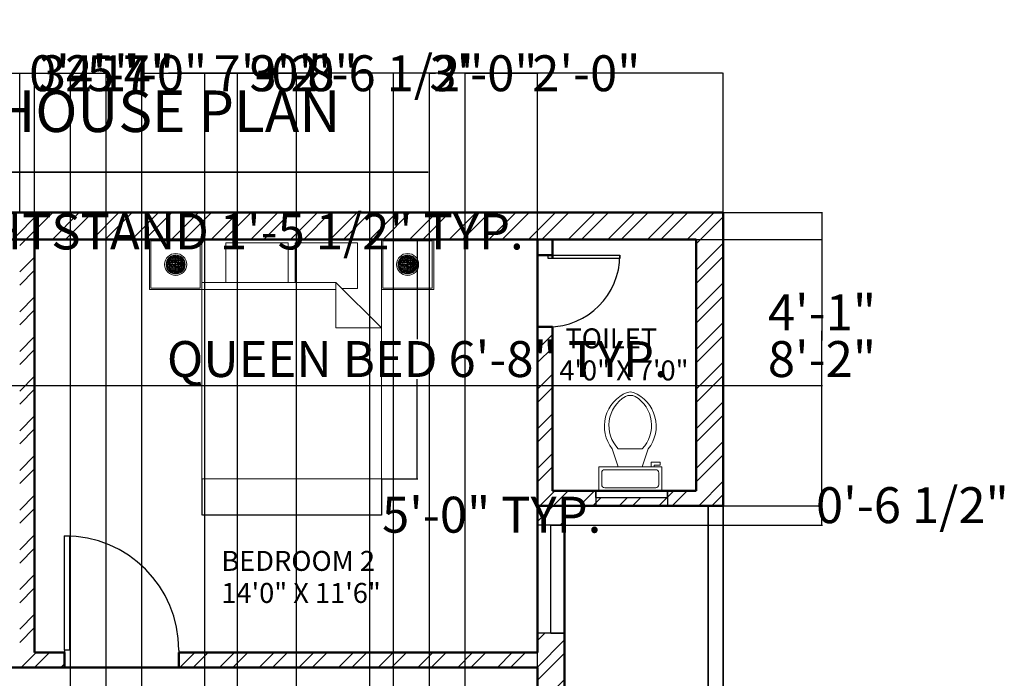
# Model space of a CAD drawing. Units: inches. Extents: x -40 to 578, y -482 to 237.
# Tile 7 of 7: x 249 to 578, y 17 to 237. Entities that reach past the tile are written whole.
import ezdxf

# ---------------------------------------------------------------- set-up
doc = ezdxf.new("R2010")
doc.units = ezdxf.units.IN
doc.header["$MEASUREMENT"] = 0
for name, color, linetype, lineweight in [('A-ANNO-DIMS', 2, 'Continuous', 18), ('A-ANNO-TEXT', 7, 'Continuous', 35), ('A-AREA-IDEN', 240, 'Continuous', 25), ('A-FLOR-FIXT', 4, 'Continuous', 18), ('A-FURN', 4, 'Continuous', 18), ('A-WALL-PATT', 252, 'Continuous', 13), ('C-PROP', 3, 'Continuous', 35), ('DOORS', 2, 'Continuous', 25), ('WALLS', 3, 'Continuous', 50), ('WINDOWS', 241, 'Continuous', 25)]:
    doc.layers.add(name, color=color, linetype=linetype, lineweight=lineweight)
doc.styles.get("Standard").update_dxf_attribs({"font": 'arial.ttf'})
doc.dimstyles.get("Standard").update_dxf_attribs({"dimtxt": 12, "dimasz": 0.18, "dimexe": 0.18, "dimexo": 0.0625, "dimgap": 0.09, "dimtad": 0, "dimtih": 1, "dimtoh": 1, "dimdec": 0, "dimzin": 0, "dimdsep": 46, "dimlunit": 3, "dimtxsty": 'Standard', "dimcen": 0.09, "dimadec": 0, "dimazin": 0, "dimtfac": 1, "dimtdec": 0, "dimtofl": 0, "dimtmove": 0, "dimatfit": 3, "dimfxl": 1, "dimtolj": 1, "dimtzin": 0, "dimarcsym": 0})

# ---------------------------------------------------------------- blocks, each defined once
blk = doc.blocks.new('Bed - Queen')
for p, q in [((0, -80.00003), (0, 0)), ((0, 0), (59.99999, 0)), ((59.99999, 0), (59.99999, -80.00003)), ((7.99999, -1.2), (28.79998, -1.2)), ((7.99999, -14.4), (7.99999, -1.2)), ((28.79998, -1.2), (28.79998, -14.4)), ((31.19999, -1.2), (51.99999, -1.2)), ((31.19999, -14.4), (31.19999, -1.2)), ((51.99999, -1.2), (51.99999, -16.4)), ((0, -14.4), (44.8, -14.4)), ((59.99999, -29.6), (44.8, -14.4)), ((44.8, -14.4), (44.8, -29.6)), ((51.99999, -16.4), (46.79936, -16.4)), ((44.8, -16.8), (0, -16.8)), ((44.8, -29.6), (59.99999, -29.6)), ((59.99999, -80.00003), (0, -80.00003))]:
    blk.add_line(p, q)
blk = doc.blocks.new('Toilet - top')
for p, q in [((9.5, -6), (9.5, -2)), ((-10, -8.5), (-8, -8.5)), ((-10, -9.5), (-10, -8.5)), ((-7, -9.5), (-10, -9.5)), ((-8, -8.5), (-8, -8)), ((-7, -8), (-7, -9.5)), ((-4, -8), (-6, -14)), ((4, -8), (6, -14)), ((4, -14), (-4, -14))]:
    blk.add_line(p, q)
blk.add_lwpolyline([(10.5, -8), (10.5, 0), (-10.5, 0), (-10.5, -8)], close=True)
for points in [[(-9.5, -2), (-9.5, -6)], [(8.5, -1), (-8.5, -1)], [(-8.5, -7), (8.5, -7)]]:
    blk.add_lwpolyline(points)
for centre, radius, start, end in [((-8.62, -1.88), 0.884, 81.8699, 188.1301), ((8.62, -1.88), 0.884, 351.8699, 98.1301), ((-8.62, -6.12), 0.884, 171.8699, 278.1301), ((8.62, -6.12), 0.884, 261.8699, 8.1301), ((3.52, -21.58), 12.17, 141.4691, 247.9714), ((4.2, -21.82), 11.33, 136.3677, 238.9468), ((-3.52, -21.58), 12.17, 292.0284, 38.5307), ((-4.2, -21.82), 11.33, 301.053, 43.6321), ((0, -27.88), 4, 245.7318, 294.2682), ((0, -29), 4, 254.8605, 285.1395)]:
    blk.add_arc(centre, radius, start, end)
blk = doc.blocks.new('*U10')
for p, q in [((0, 0), (0, -6)), ((40, 0), (40, -6))]:
    blk.add_line(p, q)
blk.add_lwpolyline([(0, 0), (0, 40), (1.75, 40), (1.75, 0)], close=True)
blk.add_arc((0, 0), 40, 0, 90)
blk = doc.blocks.new('NIGHTSTAND-LAMP')
for p, q in [((6.65, 10.79), (5.56, 8.46)), ((7.17, 11.17), (5.64, 7.78)), ((6.14, 10.22), (5.64, 9.09)), ((7.58, 11.36), (5.82, 7.16)), ((8.24, 11.54), (6.14, 6.59)), ((6.14, 10.22), (11.36, 10.22)), ((6.14, 10.22), (6.14, 6.58)), ((6.5, 10.65), (10.99, 10.65)), ((8.75, 11.58), (6.65, 6.01)), ((6.65, 10.79), (6.65, 6.01)), ((9.21, 11.55), (7.17, 5.63)), ((7.17, 11.17), (10.32, 11.17)), ((7.17, 11.17), (7.17, 5.63)), ((9.71, 11.43), (7.58, 5.44)), ((7.58, 11.36), (7.58, 5.44)), ((8.24, 11.54), (8.24, 5.18)), ((10.22, 11.22), (8.24, 5.26)), ((8.75, 11.58), (8.75, 5.22)), ((10.75, 10.87), (8.75, 5.22)), ((9.21, 11.55), (9.21, 5.18)), ((10.99, 10.65), (9.21, 5.18)), ((9.71, 11.43), (9.71, 5.37)), ((11.15, 10.48), (9.71, 5.37)), ((10.22, 11.22), (10.22, 5.58)), ((11.36, 10.22), (10.22, 5.58)), ((10.75, 10.87), (10.75, 5.93)), ((11.15, 10.48), (11.15, 6.31)), ((5.56, 8.4), (11.93, 8.4)), ((5.63, 7.78), (11.87, 7.78)), ((5.64, 9.09), (11.85, 9.09)), ((5.64, 9.09), (5.64, 7.71)), ((5.82, 7.16), (11.68, 7.16)), ((5.83, 9.68), (11.66, 9.68)), ((6.13, 6.59), (11.37, 6.59)), ((11.66, 9.68), (10.75, 5.93)), ((11.85, 9.09), (11.15, 6.31)), ((11.81, 9.26), (11.81, 7.54)), ((6.6, 6.05), (10.9, 6.05)), ((7.18, 5.63), (10.31, 5.63))]:
    blk.add_line(p, q)
for points in [[(17.49, 16.8), (0, 16.8), (0, 0), (17.49, 0)], [(16.99, 16.3), (0.5, 16.3), (0.5, 0.5), (16.99, 0.5)]]:
    blk.add_lwpolyline(points, close=True)
for radius in [3.68, 3.18]:
    blk.add_circle((8.75, 8.4), radius)
blk = doc.blocks.new('WIN-36IN')
for p, q in [((9, 36), (0, 36)), ((4.5, 0), (4.5, 36)), ((4.5, 36), (9, 36)), ((9, 0), (0, 0)), ((4.5, 0), (9, 0))]:
    blk.add_line(p, q)
blk = doc.blocks.new('*D28')
at = {"layer": 'A-ANNO-DIMS', "color": 0, "lineweight": -2, "transparency": 16777216}
for p, q in [((188.56, 163.51), (188.56, 166.25)), ((188.74, 166.07), (205.87, 166.07)), ((206.05, 163.51), (206.05, 166.25)), ((206.05, 166.07), (206.23, 166.07))]:
    blk.add_line(p, q, dxfattribs=at)
at = {"layer": 'A-ANNO-DIMS', "color": 0, "transparency": 16777216}
for points in [[(188.74, 166.1), (188.74, 166.04), (188.56, 166.07)], [(205.87, 166.1), (205.87, 166.04), (206.05, 166.07)]]:
    blk.add_solid(points, dxfattribs=at)
at = {"layer": 'Defpoints', "color": 0, "transparency": 16777216}
for p in [(206.05, 166.07), (188.56, 163.45), (206.05, 163.45)]:
    blk.add_point(p, dxfattribs=at)
at = {"layer": 'A-ANNO-DIMS', "color": 0, "transparency": 16777216, "insert": (313.4, 166.07), "char_height": 12, "attachment_point": 5}
blk.add_mtext('\\A1;NIGHTSTAND 1\'-5 1/2" TYP.', dxfattribs=at)
blk = doc.blocks.new('*D32')
at = {"layer": 'A-ANNO-DIMS', "color": 0, "lineweight": -2, "transparency": 16777216}
for p, q in [((369.65, 163.45), (381.77, 163.45)), ((381.59, 163.27), (381.59, 130.11)), ((381.59, 83.63), (381.59, 116.78)), ((369.65, 83.45), (381.77, 83.45))]:
    blk.add_line(p, q, dxfattribs=at)
at = {"layer": 'A-ANNO-DIMS', "color": 0, "transparency": 16777216}
for points in [[(381.56, 163.27), (381.62, 163.27), (381.59, 163.45)], [(381.56, 83.63), (381.62, 83.63), (381.59, 83.45)]]:
    blk.add_solid(points, dxfattribs=at)
at = {"layer": 'Defpoints', "color": 0, "transparency": 16777216}
for p in [(369.59, 163.45), (381.59, 163.45), (369.59, 83.45)]:
    blk.add_point(p, dxfattribs=at)
at = {"layer": 'A-ANNO-DIMS', "color": 0, "transparency": 16777216, "insert": (381.59, 123.45), "char_height": 12, "attachment_point": 5}
blk.add_mtext('\\A1;QUEEN BED 6\'-8" TYP.', dxfattribs=at)
blk = doc.blocks.new('*D33')
at = {"layer": 'A-ANNO-DIMS', "color": 0, "lineweight": -2, "transparency": 16777216}
for p, q in [((309.59, 83.38), (309.59, 71.27)), ((369.59, 83.38), (369.59, 71.27)), ((309.77, 71.45), (369.41, 71.45)), ((369.59, 71.45), (369.77, 71.45))]:
    blk.add_line(p, q, dxfattribs=at)
at = {"layer": 'A-ANNO-DIMS', "color": 0, "transparency": 16777216}
for points in [[(309.77, 71.48), (309.77, 71.42), (309.59, 71.45)], [(369.41, 71.48), (369.41, 71.42), (369.59, 71.45)]]:
    blk.add_solid(points, dxfattribs=at)
at = {"layer": 'Defpoints', "color": 0, "transparency": 16777216}
for p in [(309.59, 83.45), (369.59, 83.45), (369.59, 71.45)]:
    blk.add_point(p, dxfattribs=at)
at = {"layer": 'A-ANNO-DIMS', "color": 0, "transparency": 16777216, "insert": (406.43, 71.45), "char_height": 12, "attachment_point": 5}
blk.add_mtext('\\A1;5\'-0" TYP.', dxfattribs=at)
blk = doc.blocks.new('*D45')
at = {"layer": 'A-ANNO-DIMS', "color": 0, "lineweight": -2, "transparency": 16777216}
for p, q in [((71.74, 172.51), (71.74, 219.12)), ((71.92, 218.94), (257.04, 218.94)), ((483.56, 218.94), (298.43, 218.94)), ((483.74, 172.51), (483.74, 219.12))]:
    blk.add_line(p, q, dxfattribs=at)
at = {"layer": 'A-ANNO-DIMS', "color": 0, "transparency": 16777216}
for points in [[(71.92, 218.97), (71.92, 218.91), (71.74, 218.94)], [(483.56, 218.97), (483.56, 218.91), (483.74, 218.94)]]:
    blk.add_solid(points, dxfattribs=at)
at = {"layer": 'Defpoints', "color": 0, "transparency": 16777216}
for p in [(483.74, 218.94), (71.74, 172.45), (483.74, 172.45)]:
    blk.add_point(p, dxfattribs=at)
at = {"layer": 'A-ANNO-DIMS', "color": 0, "transparency": 16777216, "insert": (277.74, 218.94), "char_height": 12, "attachment_point": 5}
blk.add_mtext('\\A1;34\'-4"', dxfattribs=at)
blk = doc.blocks.new('*D46')
at = {"layer": 'A-ANNO-DIMS', "color": 0, "lineweight": -2, "transparency": 16777216}
for p, q in [((483.8, 172.45), (516.97, 172.45)), ((516.79, 172.27), (516.79, 129.66)), ((516.79, 74.63), (516.79, 117.23)), ((483.8, 74.45), (516.97, 74.45))]:
    blk.add_line(p, q, dxfattribs=at)
at = {"layer": 'A-ANNO-DIMS', "color": 0, "transparency": 16777216}
for points in [[(516.76, 172.27), (516.82, 172.27), (516.79, 172.45)], [(516.76, 74.63), (516.82, 74.63), (516.79, 74.45)]]:
    blk.add_solid(points, dxfattribs=at)
at = {"layer": 'Defpoints', "color": 0, "transparency": 16777216}
for p in [(483.74, 172.45), (516.79, 172.45), (483.74, 74.45)]:
    blk.add_point(p, dxfattribs=at)
at = {"layer": 'A-ANNO-DIMS', "color": 0, "transparency": 16777216, "insert": (516.79, 123.45), "char_height": 12, "attachment_point": 5}
blk.add_mtext('\\A1;8\'-2"', dxfattribs=at)
blk = doc.blocks.new('*D49')
at = {"layer": 'A-ANNO-DIMS', "color": 0, "lineweight": -2, "transparency": 16777216}
for p, q in [((385.66, -377.49), (385.66, 219.12)), ((385.84, 218.94), (387.66, 218.94)), ((421.56, 218.94), (419.73, 218.94)), ((421.74, -377.49), (421.74, 219.12))]:
    blk.add_line(p, q, dxfattribs=at)
at = {"layer": 'A-ANNO-DIMS', "color": 0, "transparency": 16777216}
for points in [[(385.84, 218.97), (385.84, 218.91), (385.66, 218.94)], [(421.56, 218.97), (421.56, 218.91), (421.74, 218.94)]]:
    blk.add_solid(points, dxfattribs=at)
at = {"layer": 'Defpoints', "color": 0, "transparency": 16777216}
for p in [(421.74, 218.94), (385.66, -377.55), (421.74, -377.55)]:
    blk.add_point(p, dxfattribs=at)
at = {"layer": 'A-ANNO-DIMS', "color": 0, "transparency": 16777216, "insert": (403.7, 218.94), "char_height": 12, "attachment_point": 5}
blk.add_mtext('\\A1;3\'-0"', dxfattribs=at)
blk = doc.blocks.new('*D50')
at = {"layer": 'A-ANNO-DIMS', "color": 0, "lineweight": -2, "transparency": 16777216}
for p, q in [((265.66, -330.99), (265.66, 219.12)), ((265.84, 218.94), (277.48, 218.94)), ((277.66, -330.99), (277.66, 219.12)), ((277.66, 218.94), (277.84, 218.94))]:
    blk.add_line(p, q, dxfattribs=at)
at = {"layer": 'A-ANNO-DIMS', "color": 0, "transparency": 16777216}
for points in [[(265.84, 218.97), (265.84, 218.91), (265.66, 218.94)], [(277.48, 218.97), (277.48, 218.91), (277.66, 218.94)]]:
    blk.add_solid(points, dxfattribs=at)
at = {"layer": 'Defpoints', "color": 0, "transparency": 16777216}
for p in [(277.66, 218.94), (265.66, -331.05), (277.66, -331.05)]:
    blk.add_point(p, dxfattribs=at)
at = {"layer": 'A-ANNO-DIMS', "color": 0, "transparency": 16777216, "insert": (293.31, 218.94), "char_height": 12, "attachment_point": 5}
blk.add_mtext('\\A1;1\'-0"', dxfattribs=at)
blk = doc.blocks.new('*D52')
at = {"layer": 'A-ANNO-DIMS', "color": 0, "lineweight": -2, "transparency": 16777216}
for p, q in [((234.57, -377.49), (234.57, 219.12)), ((234.75, 218.94), (265.48, 218.94)), ((265.66, -377.49), (265.66, 219.12)), ((265.66, 218.94), (265.84, 218.94))]:
    blk.add_line(p, q, dxfattribs=at)
at = {"layer": 'A-ANNO-DIMS', "color": 0, "transparency": 16777216}
for points in [[(234.75, 218.97), (234.75, 218.91), (234.57, 218.94)], [(265.48, 218.97), (265.48, 218.91), (265.66, 218.94)]]:
    blk.add_solid(points, dxfattribs=at)
at = {"layer": 'Defpoints', "color": 0, "transparency": 16777216}
for p in [(265.66, 218.94), (234.57, -377.55), (265.66, -377.55)]:
    blk.add_point(p, dxfattribs=at)
at = {"layer": 'A-ANNO-DIMS', "color": 0, "transparency": 16777216, "insert": (281.98, 218.94), "char_height": 12, "attachment_point": 5}
blk.add_mtext('\\A1;2\'-7"', dxfattribs=at)
blk = doc.blocks.new('*D61')
at = {"layer": 'A-ANNO-DIMS', "color": 0, "lineweight": -2, "transparency": 16777216}
for p, q in [((248.74, 172.51), (248.74, 219.12)), ((248.92, 218.94), (253.56, 218.94)), ((253.74, 172.51), (253.74, 219.12)), ((253.74, 218.94), (253.92, 218.94))]:
    blk.add_line(p, q, dxfattribs=at)
at = {"layer": 'A-ANNO-DIMS', "color": 0, "transparency": 16777216}
for points in [[(248.92, 218.97), (248.92, 218.91), (248.74, 218.94)], [(253.56, 218.97), (253.56, 218.91), (253.74, 218.94)]]:
    blk.add_solid(points, dxfattribs=at)
at = {"layer": 'Defpoints', "color": 0, "transparency": 16777216}
for p in [(253.74, 218.94), (248.74, 172.45), (253.74, 172.45)]:
    blk.add_point(p, dxfattribs=at)
at = {"layer": 'A-ANNO-DIMS', "color": 0, "transparency": 16777216, "insert": (269.96, 218.94), "char_height": 12, "attachment_point": 5}
blk.add_mtext('\\A1;0\'-5"', dxfattribs=at)
blk = doc.blocks.new('*D62')
at = {"layer": 'A-ANNO-DIMS', "color": 0, "lineweight": -2, "transparency": 16777216}
for p, q in [((80.8, 163.45), (516.97, 163.45)), ((516.79, 163.27), (516.79, 145.16)), ((516.79, 114.81), (516.79, 132.93)), ((80.8, 114.63), (516.97, 114.63))]:
    blk.add_line(p, q, dxfattribs=at)
at = {"layer": 'A-ANNO-DIMS', "color": 0, "transparency": 16777216}
for points in [[(516.76, 163.27), (516.82, 163.27), (516.79, 163.45)], [(516.76, 114.81), (516.82, 114.81), (516.79, 114.63)]]:
    blk.add_solid(points, dxfattribs=at)
at = {"layer": 'Defpoints', "color": 0, "transparency": 16777216}
for p in [(80.74, 163.45), (80.74, 114.63), (516.79, 114.63)]:
    blk.add_point(p, dxfattribs=at)
at = {"layer": 'A-ANNO-DIMS', "color": 0, "transparency": 16777216, "insert": (516.79, 139.04), "char_height": 12, "attachment_point": 5}
blk.add_mtext('\\A1;4\'-1"', dxfattribs=at)
blk = doc.blocks.new('*D63')
at = {"layer": 'A-ANNO-DIMS', "color": 0, "lineweight": -2, "transparency": 16777216}
for p, q in [((289.56, -104.49), (289.56, 219.12)), ((289.74, 218.94), (327.56, 218.94)), ((397.45, 218.94), (359.64, 218.94)), ((397.63, -104.49), (397.63, 219.12))]:
    blk.add_line(p, q, dxfattribs=at)
at = {"layer": 'A-ANNO-DIMS', "color": 0, "transparency": 16777216}
for points in [[(289.74, 218.97), (289.74, 218.91), (289.56, 218.94)], [(397.45, 218.97), (397.45, 218.91), (397.63, 218.94)]]:
    blk.add_solid(points, dxfattribs=at)
at = {"layer": 'Defpoints', "color": 0, "transparency": 16777216}
for p in [(397.63, 218.94), (289.56, -104.55), (397.63, -104.55)]:
    blk.add_point(p, dxfattribs=at)
at = {"layer": 'A-ANNO-DIMS', "color": 0, "transparency": 16777216, "insert": (343.6, 218.94), "char_height": 12, "attachment_point": 5}
blk.add_mtext('\\A1;9\'-0"', dxfattribs=at)
blk = doc.blocks.new('*D64')
at = {"layer": 'A-ANNO-DIMS', "color": 0, "lineweight": -2, "transparency": 16777216}
for p, q in [((397.63, -36.81), (397.63, 219.12)), ((397.81, 218.94), (421.56, 218.94)), ((421.74, -36.81), (421.74, 219.12)), ((421.74, 218.94), (421.92, 218.94))]:
    blk.add_line(p, q, dxfattribs=at)
at = {"layer": 'A-ANNO-DIMS', "color": 0, "transparency": 16777216}
for points in [[(397.81, 218.97), (397.81, 218.91), (397.63, 218.94)], [(421.56, 218.97), (421.56, 218.91), (421.74, 218.94)]]:
    blk.add_solid(points, dxfattribs=at)
at = {"layer": 'Defpoints', "color": 0, "transparency": 16777216}
for p in [(421.74, 218.94), (397.63, -36.87), (421.74, -36.87)]:
    blk.add_point(p, dxfattribs=at)
at = {"layer": 'A-ANNO-DIMS', "color": 0, "transparency": 16777216, "insert": (438.06, 218.94), "char_height": 12, "attachment_point": 5}
blk.add_mtext('\\A1;2\'-0"', dxfattribs=at)
blk = doc.blocks.new('*D67')
at = {"layer": 'A-ANNO-DIMS', "color": 0, "lineweight": -2, "transparency": 16777216}
for p, q in [((321.5, -108), (321.5, 219.12)), ((321.68, 218.94), (327.57, 218.94)), ((365.53, 218.94), (359.64, 218.94)), ((365.71, -108), (365.71, 219.12))]:
    blk.add_line(p, q, dxfattribs=at)
at = {"layer": 'A-ANNO-DIMS', "color": 0, "transparency": 16777216}
for points in [[(321.68, 218.97), (321.68, 218.91), (321.5, 218.94)], [(365.53, 218.97), (365.53, 218.91), (365.71, 218.94)]]:
    blk.add_solid(points, dxfattribs=at)
at = {"layer": 'Defpoints', "color": 0, "transparency": 16777216}
for p in [(365.71, 218.94), (321.5, -108.06), (365.71, -108.06)]:
    blk.add_point(p, dxfattribs=at)
at = {"layer": 'A-ANNO-DIMS', "color": 0, "transparency": 16777216, "insert": (343.6, 218.94), "char_height": 12, "attachment_point": 5}
blk.add_mtext('\\A1;3\'-8"', dxfattribs=at)
blk = doc.blocks.new('*D73')
at = {"layer": 'A-ANNO-DIMS', "color": 0, "lineweight": -2, "transparency": 16777216}
for p, q in [((289.59, -268.55), (289.59, 219.12)), ((289.77, 218.94), (315.6, 218.94)), ((373.41, 218.94), (347.58, 218.94)), ((373.59, -268.55), (373.59, 219.12))]:
    blk.add_line(p, q, dxfattribs=at)
at = {"layer": 'A-ANNO-DIMS', "color": 0, "transparency": 16777216}
for points in [[(289.77, 218.97), (289.77, 218.91), (289.59, 218.94)], [(373.41, 218.97), (373.41, 218.91), (373.59, 218.94)]]:
    blk.add_solid(points, dxfattribs=at)
at = {"layer": 'Defpoints', "color": 0, "transparency": 16777216}
for p in [(373.59, 218.94), (289.59, -268.61), (373.59, -268.61)]:
    blk.add_point(p, dxfattribs=at)
at = {"layer": 'A-ANNO-DIMS', "color": 0, "transparency": 16777216, "insert": (331.59, 218.94), "char_height": 12, "attachment_point": 5}
blk.add_mtext('\\A1;7\'-0"', dxfattribs=at)
blk = doc.blocks.new('*D75')
at = {"layer": 'A-ANNO-DIMS', "color": 0, "lineweight": -2, "transparency": 16777216}
for p, q in [((310.54, -218.11), (310.54, 219.12)), ((310.72, 218.94), (340.99, 218.94)), ((341.17, -218.11), (341.17, 219.12)), ((341.17, 218.94), (341.35, 218.94))]:
    blk.add_line(p, q, dxfattribs=at)
at = {"layer": 'A-ANNO-DIMS', "color": 0, "transparency": 16777216}
for points in [[(310.72, 218.97), (310.72, 218.91), (310.54, 218.94)], [(340.99, 218.97), (340.99, 218.91), (341.17, 218.94)]]:
    blk.add_solid(points, dxfattribs=at)
at = {"layer": 'Defpoints', "color": 0, "transparency": 16777216}
for p in [(341.17, 218.94), (310.54, -218.17), (341.17, -218.17)]:
    blk.add_point(p, dxfattribs=at)
at = {"layer": 'A-ANNO-DIMS', "color": 0, "transparency": 16777216, "insert": (371.48, 218.94), "char_height": 12, "attachment_point": 5}
blk.add_mtext('\\A1;2\'-6 1/2"', dxfattribs=at)
blk = doc.blocks.new('*D77')
at = {"layer": 'A-ANNO-DIMS', "color": 0, "lineweight": -2, "transparency": 16777216}
for p, q in [((430.8, 74.45), (516.97, 74.45)), ((516.79, 74.45), (516.79, 74.63)), ((516.79, 74.63), (516.97, 74.63)), ((516.79, 68.08), (516.79, 74.27)), ((430.8, 67.9), (516.97, 67.9))]:
    blk.add_line(p, q, dxfattribs=at)
at = {"layer": 'A-ANNO-DIMS', "color": 0, "transparency": 16777216}
for points in [[(516.76, 74.27), (516.82, 74.27), (516.79, 74.45)], [(516.76, 68.08), (516.82, 68.08), (516.79, 67.9)]]:
    blk.add_solid(points, dxfattribs=at)
at = {"layer": 'Defpoints', "color": 0, "transparency": 16777216}
for p in [(430.74, 74.45), (516.79, 74.45), (430.74, 67.9)]:
    blk.add_point(p, dxfattribs=at)
at = {"layer": 'A-ANNO-DIMS', "color": 0, "transparency": 16777216, "insert": (546.99, 74.63), "char_height": 12, "attachment_point": 5}
blk.add_mtext('\\A1;0\'-6 1/2"', dxfattribs=at)

msp = doc.modelspace()

# ---------------------------------------------------------------- hatches: boundary and pattern name
at = {"layer": 'A-WALL-PATT'}
h = msp.add_hatch(dxfattribs=at)
h.set_pattern_fill('ANSI32', color=256, scale=25)
h.set_pattern_definition([(45, (-1993.713, -1175.095), (-6.629126, 6.629126), []), (45, (-1989.294, -1175.095), (-6.629126, 6.629126), [])])
h.paths.add_polyline_path([(248.74, 172.45), (71.74, 172.45), (71.74, 114.63), (80.74, 114.63), (80.74, 163.45), (248.74, 163.45)])
h.paths.add_polyline_path([(253.74, 172.45), (248.74, 172.45), (248.74, 163.45), (253.74, 163.45)])
h.paths.add_polyline_path([(253.74, 163.45), (248.74, 163.45), (248.74, 25.45), (240.62, 25.45), (240.62, 20.45), (263.71, 20.45), (263.71, 25.45), (253.74, 25.45)])
h.paths.add_polyline_path([(483.74, 172.45), (253.74, 172.45), (253.74, 163.45), (426.74, 163.45), (474.74, 163.45), (474.74, 79.45), (465.23, 79.45), (465.23, 77.2), (441.23, 77.2), (441.23, 74.45), (483.74, 74.45)])
h.paths.add_polyline_path([(80.74, 78.63), (71.74, 78.63), (71.74, 3.32), (80.74, 3.32), (80.74, 20.45), (134.6, 20.45), (134.6, 25.45), (80.74, 25.45)])
h.paths.add_polyline_path([(202.4, 25.45), (158.53, 25.45), (158.53, 20.45), (202.4, 20.45)])
h.paths.add_polyline_path([(169.74, 20.45), (164.74, 20.45), (164.74, -39.55), (80.74, -39.55), (80.74, -20.68), (71.74, -20.68), (71.74, -61.38), (80.74, -61.38), (80.74, -44.55), (164.74, -44.55), (164.74, -104.55), (169.74, -104.55), (169.74, -44.55)])
h.paths.add_polyline_path([(135.96, -104.55), (80.74, -104.55), (80.74, -85.38), (71.74, -85.38), (71.74, -155.89), (80.74, -155.89), (80.74, -109.55), (135.96, -109.55)])
h.paths.add_polyline_path([(218.74, -104.55), (159.9, -104.55), (159.9, -109.55), (218.74, -109.55)])
h.paths.add_polyline_path([(223.74, -104.55), (218.74, -104.55), (218.74, -109.55), (223.74, -109.55)])
h.paths.add_polyline_path([(223.74, -109.55), (218.74, -109.55), (218.74, -114.58), (223.74, -114.58)])
h.paths.add_polyline_path([(430.74, -85.66), (421.74, -85.66), (421.74, -128.55), (223.74, -128.55), (223.74, -133.55), (421.74, -133.55), (421.74, -197.77), (430.74, -197.77)])
h.paths.add_polyline_path([(223.74, -152.8), (218.74, -152.8), (218.74, -229.55), (151.59, -229.55), (151.59, -238.55), (223.74, -238.55), (223.74, -229.55)])
h.paths.add_polyline_path([(115.59, -229.55), (98.23, -229.55), (80.74, -229.55), (80.74, -212.75), (80.74, -191.89), (71.74, -191.89), (71.74, -238.55), (115.59, -238.55)])
h.paths.add_polyline_path([(307.53, -289.55), (223.74, -289.55), (223.74, -283.47), (218.74, -283.47), (218.74, -298.55), (307.53, -298.55)])
h.paths.add_polyline_path([(421.74, -289.55), (343.53, -289.55), (343.53, -298.55), (421.74, -298.55)])
h.paths.add_polyline_path([(430.74, -367.34), (421.74, -367.34), (421.74, -377.55), (234.57, -377.55), (234.57, -386.55), (430.74, -386.55)])
h.paths.add_polyline_path([(430.74, -298.55), (430.74, -233.77), (421.74, -233.77), (421.74, -289.55), (421.74, -298.55), (421.74, -331.34), (430.74, -331.34)])
h.paths.add_polyline_path([(430.74, -11.67), (427.15, -11.67, -0.057068), (421.74, -11.05), (421.74, -49.66), (430.74, -49.66)])
h.paths.add_polyline_path([(430.74, 31.9), (421.74, 31.9), (421.74, 25.45), (301.93, 25.45), (301.93, 20.45), (421.74, 20.45), (421.74, 12.26), (430.74, 12.26)])
h.paths.add_polyline_path([(426.74, 134.23, -0.014739), (425.33, 134.19), (421.74, 134.19), (421.74, 74.45), (441.23, 74.45), (441.23, 77.2), (441.23, 79.45), (426.74, 79.45)], flags=17)
h.paths.add_polyline_path([(430.74, 74.45), (421.74, 74.45), (421.74, 67.9), (430.74, 67.9)])

# ---------------------------------------------------------------- linework, layer by layer
at = {"layer": 'A-ANNO-TEXT'}
msp.add_line((133.78, 185.89), (385.18, 185.89), dxfattribs=at)
at = {"layer": 'C-PROP'}
for p, q in [((478.74, 74.45), (478.74, -432.55)), ((483.74, 74.45), (483.74, -441.55))]:
    msp.add_line(p, q, dxfattribs=at)
at = {"layer": 'WALLS'}
for p, q in [((483.74, 172.45), (71.74, 172.45)), ((253.74, 172.45), (253.74, 25.45)), ((483.74, 172.45), (483.74, 74.45)), ((426.74, 163.45), (80.74, 163.45)), ((421.74, 163.45), (421.74, 25.45)), ((426.74, 163.45), (426.74, 157.07)), ((426.74, 163.45), (474.74, 163.45)), ((474.74, 163.45), (474.74, 79.45)), ((421.74, 158.12), (426.74, 158.12)), ((421.74, 134.19), (426.74, 134.23)), ((426.74, 134.23), (426.74, 79.45)), ((426.74, 79.45), (474.74, 79.45)), ((421.74, 74.45), (483.74, 74.45)), ((430.74, 74.45), (430.74, -298.55)), ((263.71, 25.45), (253.74, 25.45)), ((263.71, 25.45), (263.71, 20.45)), ((421.74, 25.45), (301.93, 25.45)), ((301.93, 25.45), (301.93, 20.45)), ((421.74, 20.45), (157.49, 20.45)), ((421.74, 20.45), (421.74, 11.22))]:
    msp.add_line(p, q, dxfattribs=at)
at = {"layer": 'WINDOWS'}
for p, q in [((441.23, 77.2), (441.23, 79.45)), ((441.23, 79.45), (441.23, 74.45)), ((465.23, 77.45), (465.23, 79.7)), ((465.23, 79.7), (465.23, 74.7)), ((441.23, 77.2), (465.23, 77.2))]:
    msp.add_line(p, q, dxfattribs=at)

# ---------------------------------------------------------------- block references
at = {"layer": 'A-FLOR-FIXT', "rotation": 180}
msp.add_blockref('Toilet - top', (452.74, 79.45), dxfattribs=at)
at = {"layer": 'A-FURN'}
for name, p in [('NIGHTSTAND-LAMP', (292.1, 146.65)), ('Bed - Queen', (309.59, 163.45)), ('NIGHTSTAND-LAMP', (369.59, 146.65))]:
    msp.add_blockref(name, p, dxfattribs=at)
at = {"layer": 'DOORS', "xscale": 0.5983195859330738, "yscale": 0.5983195859330738, "zscale": 0.5983195859330738, "rotation": 270}
msp.add_blockref('*U10', (425.33, 158.12), dxfattribs=at)
at = {"layer": 'DOORS', "xscale": 0.9555568703817776, "yscale": 0.9555568703817776, "zscale": 0.9555568703817776}
msp.add_blockref('*U10', (263.71, 26.18), dxfattribs=at)
at = {"layer": 'WINDOWS'}
msp.add_blockref('WIN-36IN', (421.74, 31.9), dxfattribs=at)

# ---------------------------------------------------------------- texts
at = {"layer": 'A-ANNO-TEXT'}
msp.add_text('WEST FACE HOUSE PLAN', height=13.8818, dxfattribs=at).set_placement((136.08, 199.3))
at = {"layer": 'A-AREA-IDEN'}
for s, height, p in [('   TOILET', 6.67, (424.95, 127.03)), ('  4\'0" X 7\'0"', 6.6698, (424.95, 116.32)), ('BEDROOM 2', 6.67, (316.11, 52.68)), ('14\'0" X 11\'6"', 6.6698, (316.11, 41.97))]:
    msp.add_text(s, height=height, dxfattribs=at).set_placement(p)

# ---------------------------------------------------------------- dimensions: what is measured, and where the dimension line sits
at = {"layer": 'A-ANNO-DIMS'}
for base, p1, p2, picture, middle in [((341.17, 218.94), (310.54, -218.17), (341.17, -218.17), '*D75', (371.48, 218.94)), ((483.74, 218.94), (71.74, 172.45), (483.74, 172.45), '*D45', (277.74, 218.94)), ((265.66, 218.94), (234.57, -377.55), (265.66, -377.55), '*D52', (281.98, 218.94)), ((253.74, 218.94), (248.74, 172.45), (253.74, 172.45), '*D61', (269.96, 218.94)), ((277.66, 218.94), (265.66, -331.05), (277.66, -331.05), '*D50', (293.31, 218.94)), ((397.63, 218.94), (289.56, -104.55), (397.63, -104.55), '*D63', (343.6, 218.94)), ((373.59, 218.94), (289.59, -268.61), (373.59, -268.61), '*D73', (331.59, 218.94)), ((365.71, 218.94), (321.5, -108.06), (365.71, -108.06), '*D67', (343.6, 218.94)), ((421.74, 218.94), (385.66, -377.55), (421.74, -377.55), '*D49', (403.7, 218.94)), ((421.74, 218.94), (397.63, -36.87), (421.74, -36.87), '*D64', (438.06, 218.94))]:
    dim = msp.add_linear_dim(base=base, p1=p1, p2=p2, dimstyle='Standard', override={"dimdec": 1, "dimlfac": 1, "dimrnd": 0, "dimzin": 1, "dimdsep": 46, "dimlunit": 4, "dimfrac": 2}, dxfattribs=at)
    dim.commit()
    dim.dimension.update_dxf_attribs({"geometry": picture, "text_midpoint": middle})
for base, p1, p2, text, picture, middle in [((206.05, 166.07), (188.56, 163.45), (206.05, 163.45), 'NIGHTSTAND <> TYP.', '*D28', (313.4, 166.07)), ((369.59, 71.45), (309.59, 83.45), (369.59, 83.45), '<> TYP.', '*D33', (406.43, 71.45))]:
    dim = msp.add_linear_dim(base=base, p1=p1, p2=p2, text=text, dimstyle='Standard', override={"dimdec": 1, "dimlfac": 1, "dimrnd": 0, "dimzin": 1, "dimdsep": 46, "dimlunit": 4, "dimfrac": 2}, dxfattribs=at)
    dim.commit()
    dim.dimension.update_dxf_attribs({"geometry": picture, "text_midpoint": middle})
for base, p1, p2, picture, middle in [((516.79, 172.45), (483.74, 74.45), (483.74, 172.45), '*D46', (516.79, 123.45)), ((516.79, 114.63), (80.74, 163.45), (80.74, 114.63), '*D62', (516.79, 139.04)), ((516.7877, 74.4475), (430.7377, 67.904), (430.7377, 74.4475), '*D77', (546.9881, 74.6275))]:
    dim = msp.add_linear_dim(base=base, p1=p1, p2=p2, angle=90, dimstyle='Standard', override={"dimdec": 1, "dimlfac": 1, "dimrnd": 0, "dimzin": 1, "dimdsep": 46, "dimlunit": 4, "dimfrac": 2}, dxfattribs=at)
    dim.commit()
    dim.dimension.update_dxf_attribs({"geometry": picture, "text_midpoint": middle})
dim = msp.add_linear_dim(base=(381.59, 163.45), p1=(369.59, 83.45), p2=(369.59, 163.45), angle=90, text='QUEEN BED <> TYP.', dimstyle='Standard', override={"dimdec": 1, "dimlfac": 1, "dimrnd": 0, "dimzin": 1, "dimdsep": 46, "dimlunit": 4, "dimfrac": 2}, dxfattribs=at)
dim.commit()
dim.dimension.update_dxf_attribs({"geometry": '*D32', "text_midpoint": (381.59, 123.45)})

doc.saveas('drawing.dxf')
